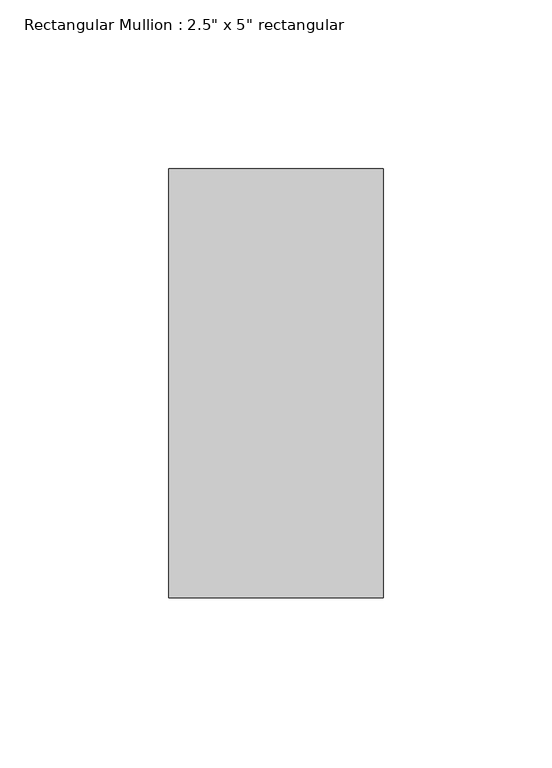
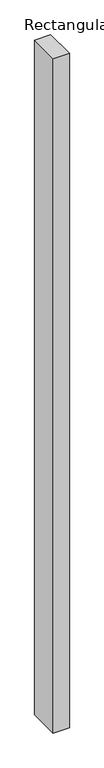
"""IFC4 building model written with IfcOpenShell, lengths in millimetres: member geometry."""

from ifc_helpers import new_model, si_unit, frame, origin, place, context, project, spatial, polyline, outline, extrude, source, transform, mapped, element, save


def member_46bdb8c2(model_context):
    return source(origin(), model_context, "Body", "SweptSolid", [
        extrude(outline(polyline([(31.75, 63.5), (31.75, -63.5), (-31.75, -63.5), (-31.75, 63.5), (31.75, 63.5)])), frame((0.0, 0.0, -2816.4340209), z_axis=(0.0, 0.0, 1.0), x_axis=(1.0, 0.0, 0.0)), (0.0, 0.0, 1.0), 2816.4340209),
    ])


if __name__ == "__main__":
    model = new_model("IFC4")
    model_context = context("Model", 3, world=origin())
    ifc_project = project(units=[si_unit("LENGTHUNIT", "METRE", prefix="MILLI")], contexts=[model_context])
    site = spatial("IfcSite", under=ifc_project)
    building = spatial("IfcBuilding", under=site)
    placement = place(None, origin())
    member_shape = member_46bdb8c2(model_context)
    element("IfcMember", 1, ObjectType="Rectangular Mullion : 2.5\" x 5\" rectangular", at=placement, inside=building, context=model_context, shape_type="MappedRepresentation", body=[
        mapped(member_shape, transform((0.0, 0.0, 0.0), x_axis=(1.0, 0.0, 0.0), y_axis=(0.0, 1.0, 0.0), z_axis=(0.0, 0.0, 1.0))),
    ])
    save(model, "model.ifc")

# Revit data of these elements
# Type "Rectangular Mullion : 2.5\" x 5\" rectangular"
#   built-in parameter 1007304 = 0.416667 (stored number, unit not read)
#   built-in parameter 1007301 = 0.104167 (stored number, unit not read)
#   built-in parameter 1007300 = 0.104167 (stored number, unit not read)
# Element 1 (IfcMember, "Rectangular Mullion : 2.5\" x 5\" rectangular")
#   Materials on its faces: "Aluminum"
# Materials
#   "Aluminum": class "Metal", colour RGB 247 247 247, transparency 0, Description = "Aluminum 6061", Cost = 0
